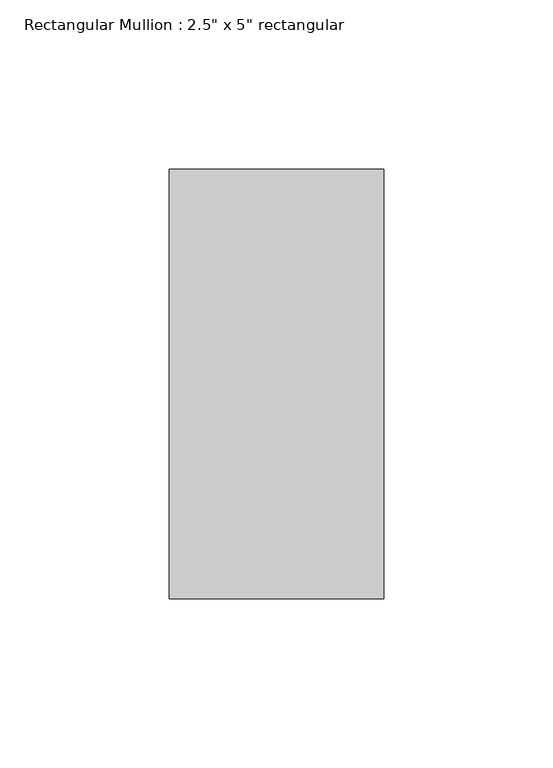
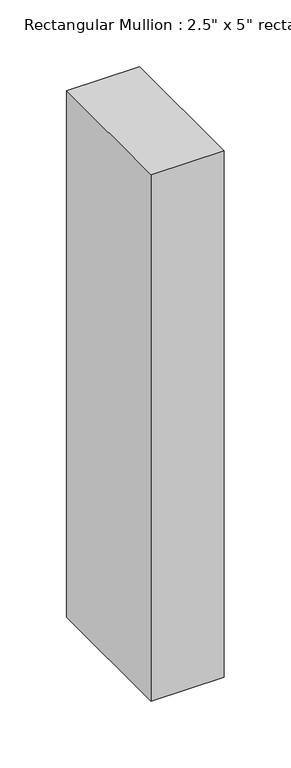
"""IFC4 building model written with IfcOpenShell, lengths in millimetres: member geometry."""

from ifc_helpers import new_model, si_unit, frame, origin, place, context, project, spatial, polyline, outline, extrude, source, transform, mapped, element, save


def member_86d06fe4(model_context):
    return source(origin(), model_context, "Body", "SweptSolid", [
        extrude(outline(polyline([(0.0, 63.5), (0.0, -63.5), (-63.5, -63.5), (-63.5, 63.5), (0.0, 63.5)])), frame((0.0, 0.0, -482.6), z_axis=(0.0, 0.0, 1.0), x_axis=(1.0, 0.0, 0.0)), (0.0, 0.0, 1.0), 482.6),
    ])


if __name__ == "__main__":
    model = new_model("IFC4")
    model_context = context("Model", 3, world=origin())
    ifc_project = project(units=[si_unit("LENGTHUNIT", "METRE", prefix="MILLI")], contexts=[model_context])
    site = spatial("IfcSite", under=ifc_project)
    building = spatial("IfcBuilding", under=site)
    placement = place(None, origin())
    member_shape = member_86d06fe4(model_context)
    element("IfcMember", 1, ObjectType="Rectangular Mullion : 2.5\" x 5\" rectangular", at=placement, inside=building, context=model_context, shape_type="MappedRepresentation", body=[
        mapped(member_shape, transform((0.0, 0.0, 0.0), x_axis=(1.0, 0.0, 0.0), y_axis=(0.0, 1.0, 0.0), z_axis=(0.0, 0.0, 1.0))),
    ])
    save(model, "model.ifc")

# Revit data of these elements
# Type "Rectangular Mullion : 2.5\" x 5\" rectangular"
#   built-in parameter 1007304 = 0.416667 (stored number, unit not read)
#   built-in parameter 1007301 = 0.104167 (stored number, unit not read)
#   built-in parameter 1007300 = 0.104167 (stored number, unit not read)
# Element 1 (IfcMember, "Rectangular Mullion : 2.5\" x 5\" rectangular")
#   Materials on its faces: "Aluminum"
# Materials
#   "Aluminum": class "Metal", colour RGB 247 247 247, transparency 0, Description = "Aluminum 6061", Cost = 0
